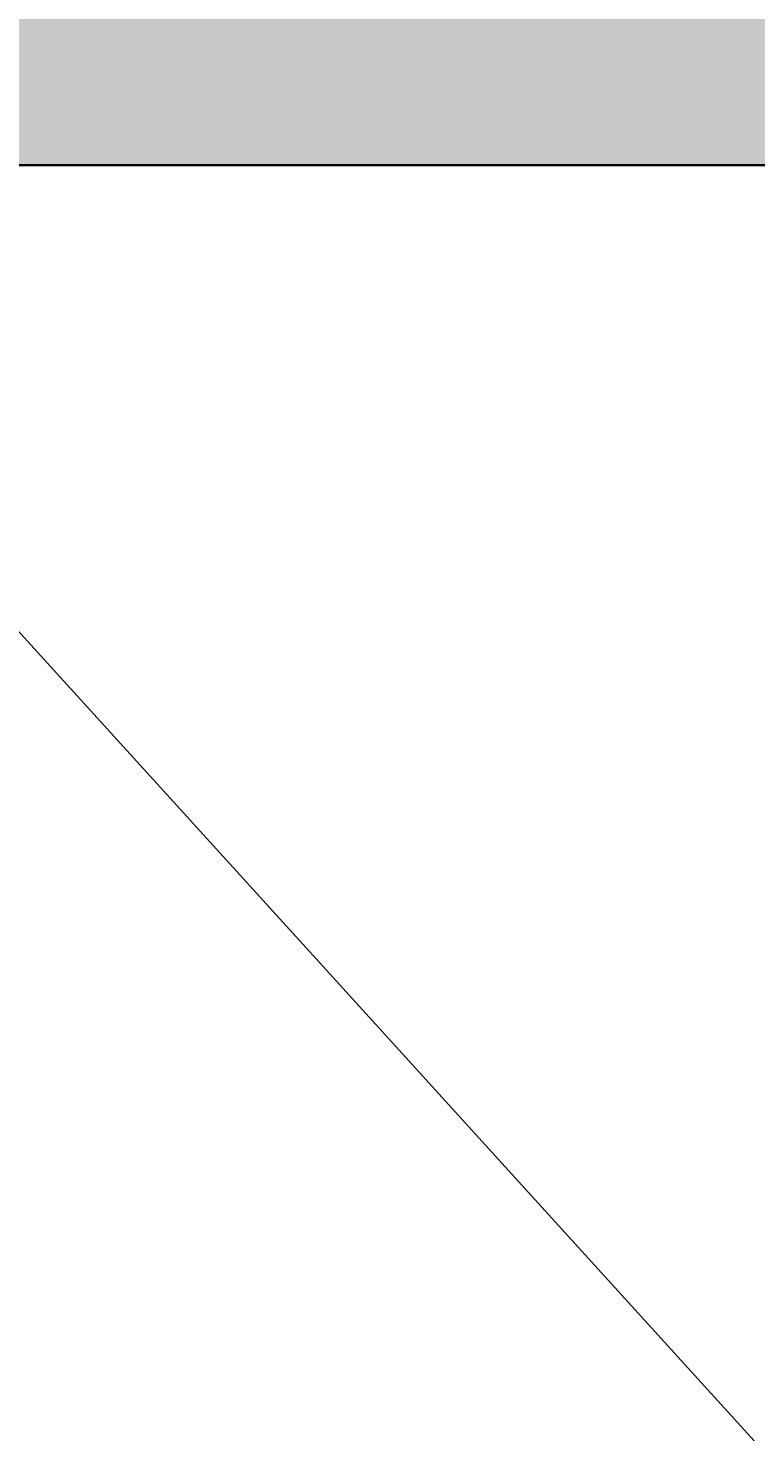
# Model space of a CAD drawing. Units: inches. Extents: x 1998 to 2588, y 1139 to 1977.
# Tile 34 of 134: x 2238 to 2257, y 1557 to 1592. Entities that reach past the tile are written whole.
import ezdxf

# ---------------------------------------------------------------- set-up
doc = ezdxf.new("R2010")
doc.units = ezdxf.units.IN
for name, color, linetype, lineweight in [('A-ANNO-DIMS', 2, 'Continuous', 18), ('A-FLOR-OPEN', 8, 'Continuous', 18), ('A-WALL-PATT', 252, 'Continuous', 13), ('WALL', 200, 'Continuous', 35)]:
    doc.layers.add(name, color=color, linetype=linetype, lineweight=lineweight)
doc.styles.get("Standard").update_dxf_attribs({"font": 'arial.ttf'})
doc.dimstyles.get("Standard").update_dxf_attribs({"dimtxt": 0.18, "dimasz": 0.18, "dimexe": 0.18, "dimexo": 0.0625, "dimgap": 0.09, "dimtad": 0, "dimtih": 1, "dimtoh": 1, "dimdec": 4, "dimzin": 0, "dimdsep": 46, "dimtxsty": 'Standard', "dimcen": 0.09, "dimadec": 0, "dimazin": 0, "dimtfac": 1, "dimtdec": 4, "dimtofl": 0, "dimtmove": 0, "dimatfit": 3, "dimfxl": 1, "dimtolj": 1, "dimtzin": 0, "dimarcsym": 0})

# ---------------------------------------------------------------- blocks, each defined once
blk = doc.blocks.new('*D34')
at = {"layer": 'A-ANNO-DIMS', "color": 0, "lineweight": -2, "transparency": 16777216}
for p, q in [((2407.91, 1594.732), (1997.843, 1594.732)), ((1998.023, 1594.552), (1998.023, 1558.913)), ((1998.023, 1522.912), (1998.023, 1558.552)), ((2407.91, 1522.732), (1997.843, 1522.732))]:
    blk.add_line(p, q, dxfattribs=at)
at = {"layer": 'A-ANNO-DIMS', "color": 0, "transparency": 16777216}
for points in [[(1997.993, 1594.552), (1998.053, 1594.552), (1998.023, 1594.732)], [(1997.993, 1522.912), (1998.053, 1522.912), (1998.023, 1522.732)]]:
    blk.add_solid(points, dxfattribs=at)
at = {"layer": 'Defpoints', "color": 0, "transparency": 16777216}
for p in [(1998.023, 1594.732), (2407.973, 1594.732), (2407.973, 1522.732)]:
    blk.add_point(p, dxfattribs=at)
at = {"layer": 'A-ANNO-DIMS', "color": 0, "transparency": 16777216, "insert": (1998.023, 1558.732), "char_height": 0.18, "attachment_point": 5}
blk.add_mtext('\\A1;72', dxfattribs=at)
blk = doc.blocks.new('*D41')
at = {"layer": 'A-ANNO-DIMS', "color": 0, "lineweight": -2, "transparency": 16777216}
for p, q in [((2227.473, 1588.67), (2227.473, 1138.602)), ((2287.473, 1588.67), (2287.473, 1138.602)), ((2227.653, 1138.782), (2257.254, 1138.782)), ((2287.293, 1138.782), (2257.692, 1138.782))]:
    blk.add_line(p, q, dxfattribs=at)
at = {"layer": 'A-ANNO-DIMS', "color": 0, "transparency": 16777216}
for points in [[(2227.653, 1138.812), (2227.653, 1138.752), (2227.473, 1138.782)], [(2287.293, 1138.812), (2287.293, 1138.752), (2287.473, 1138.782)]]:
    blk.add_solid(points, dxfattribs=at)
at = {"layer": 'Defpoints', "color": 0, "transparency": 16777216}
for p in [(2227.473, 1588.732), (2287.473, 1588.732), (2287.473, 1138.782)]:
    blk.add_point(p, dxfattribs=at)
at = {"layer": 'A-ANNO-DIMS', "color": 0, "transparency": 16777216, "insert": (2257.473, 1138.782), "char_height": 0.18, "attachment_point": 5}
blk.add_mtext('\\A1;60', dxfattribs=at)

msp = doc.modelspace()

# ---------------------------------------------------------------- hatches: boundary and pattern name
at = {"layer": 'A-WALL-PATT'}
h = msp.add_hatch(color=256, dxfattribs=at)
h.dxf.hatch_style = 1
h.paths.add_polyline_path([(2222.9729, 1888.7324), (2099.4125, 1888.7324), (2099.4125, 1879.7324), (2222.9729, 1879.7324)])
h.paths.add_polyline_path([(2096.9729, 1868.3278), (2087.9729, 1868.3278), (2087.9729, 1775.637), (2096.9729, 1775.637)])
h.paths.add_polyline_path([(2227.4729, 1868.3278), (2222.9729, 1868.3278), (2222.9729, 1774.3318), (2227.4729, 1774.3318)])
h.paths.add_polyline_path([(2188.3019, 1759.7324), (2138.6074, 1759.7324), (2099.4125, 1759.7324), (2099.4125, 1755.2324), (2176.9729, 1755.2324), (2188.3019, 1755.2324)])
h.paths.add_polyline_path([(2087.9729, 1759.7324), (2059.4729, 1759.7324), (2059.4729, 1702.7324), (2087.9729, 1702.7324), (2087.9729, 1707.2324), (2063.9729, 1707.2324), (2063.9729, 1755.2324), (2087.9729, 1755.2324)])
h.paths.add_polyline_path([(2096.9729, 1755.2324), (2087.9729, 1755.2324), (2087.9729, 1707.2324), (2096.9729, 1707.2324)])
h.paths.add_polyline_path([(2187.0461, 1707.2324), (2105.9729, 1707.2324), (2096.9729, 1707.2324), (2087.9729, 1707.2324), (2087.9729, 1702.7324), (2105.9729, 1702.7324), (2114.9729, 1702.7324), (2187.0461, 1702.7324)])
h.paths.add_polyline_path([(2181.4729, 1719.2028), (2176.9729, 1719.2028), (2176.9729, 1707.2324), (2181.4729, 1707.2324)])
h.paths.add_polyline_path([(2216.0332, 1588.7324), (2114.9729, 1588.7324), (2105.9729, 1588.7324), (2105.9729, 1584.2324), (2216.0332, 1584.2324)])
h.paths.add_polyline_path([(2077.691, 1588.7324), (2061.4729, 1588.7324), (2061.4729, 1584.2324), (2077.691, 1584.2324)])
h.paths.add_polyline_path([(2105.9729, 1588.7324), (2098.0956, 1588.7324), (2098.0956, 1584.2324), (2105.9729, 1584.2324)])
h.paths.add_polyline_path([(2114.9729, 1596.2642), (2110.1012, 1596.2642), (2105.9729, 1596.2642), (2105.9729, 1588.7324), (2114.9729, 1588.7324)])
h.paths.add_polyline_path([(2114.9729, 1584.2324), (2105.9729, 1584.2324), (2105.9729, 1580.249), (2110.1012, 1580.249), (2114.9729, 1580.249)])
h.paths.add_polyline_path([(2114.9729, 1547.7716), (2110.1012, 1547.7716, -0.0318759), (2105.9729, 1548.035), (2105.9729, 1470.2324), (2108.3775, 1470.2324), (2108.3775, 1465.7324), (2186.2943, 1465.7324), (2186.2943, 1470.2324), (2114.9729, 1470.2324)])
h.paths.add_polyline_path([(2227.4729, 1584.2324), (2222.9729, 1584.2324), (2222.9729, 1486.137), (2227.4729, 1486.137)])
h.paths.add_polyline_path([(2295.4138, 1593.2324), (2227.4729, 1593.2324), (2227.4729, 1588.7324), (2295.4138, 1588.7324), (2295.4138, 1591.8729)])
h.paths.add_polyline_path([(2345.9729, 1627.1165), (2341.4729, 1627.1165), (2341.4729, 1593.2324), (2337.2869, 1593.2324), (2337.2869, 1591.8729), (2337.2869, 1588.7324), (2345.9729, 1588.7324)])
h.paths.add_polyline_path([(2291.9729, 1588.7324), (2287.4729, 1588.7324), (2287.4729, 1522.7324), (2291.9729, 1522.7324)])
h.paths.add_polyline_path([(2291.9729, 1522.7324), (2287.4729, 1522.7324), (2227.4729, 1522.7324), (2227.4729, 1518.2324), (2291.9729, 1518.2324)])
h.paths.add_polyline_path([(2295.7347, 1519.5919), (2295.7347, 1522.7324), (2291.9729, 1522.7324), (2291.9729, 1518.2324), (2295.7347, 1518.2324)])
h.paths.add_polyline_path([(2345.9729, 1522.7324), (2337.6078, 1522.7324), (2337.6078, 1519.5919), (2337.6078, 1518.2324), (2341.4729, 1518.2324), (2341.4729, 1488.5616), (2345.9729, 1488.5616)])
h.paths.add_polyline_path([(2345.9729, 1468.1569), (2341.4729, 1468.1569), (2341.4729, 1374.2324), (2227.4729, 1374.2324), (2227.4729, 1369.7324), (2345.9729, 1369.7324)])
h.paths.add_polyline_path([(2345.9729, 1369.7324), (2341.4729, 1369.7324), (2341.4729, 1362.2324), (2345.9729, 1362.2324)])
h.paths.add_polyline_path([(2345.9729, 1317.7324), (2345.9729, 1322.2324), (2341.4729, 1322.2324), (2341.4729, 1285.137), (2345.9729, 1285.137)], flags=17)
h.paths.add_polyline_path([(2356.2096, 1322.2324), (2345.9729, 1322.2324), (2345.9729, 1317.7324), (2356.2096, 1317.7324), (2356.2096, 1319.3088)], flags=17)
h.paths.add_polyline_path([(2393.9729, 1322.2324), (2375.6999, 1322.2324), (2375.6999, 1319.3088, -0.0202458), (2375.636, 1317.7324), (2393.9729, 1317.7324)], flags=17)
h.paths.add_polyline_path([(2398.4729, 1322.2324), (2393.9729, 1322.2324), (2393.9729, 1317.7324), (2393.9729, 1237.7324), (2345.9729, 1237.7324), (2345.9729, 1264.7324), (2341.4729, 1264.7324), (2341.4729, 1228.7324), (2393.9729, 1228.7324), (2482.7412, 1228.7324), (2482.7412, 1237.7324), (2398.4729, 1237.7324), (2398.4729, 1297.1029)])
h.paths.add_polyline_path([(2398.4729, 1362.2324), (2393.9729, 1362.2324), (2393.9729, 1357.7324), (2398.4729, 1357.7324)])
h.paths.add_polyline_path([(2345.9729, 1329.7549), (2341.4729, 1329.7549), (2341.4729, 1322.2324), (2345.9729, 1322.2324)])

# ---------------------------------------------------------------- linework, layer by layer
at = {"layer": 'A-FLOR-OPEN'}
msp.add_line((2227.4729, 1588.7324), (2287.4729, 1522.7324), dxfattribs=at)
at = {"layer": 'WALL'}
msp.add_line((2295.4138, 1588.7324), (2227.4729, 1588.7324), dxfattribs=at)

# ---------------------------------------------------------------- dimensions: what is measured, and where the dimension line sits
at = {"layer": 'A-ANNO-DIMS'}
dim = msp.add_linear_dim(base=(1998.0229, 1594.7324), p1=(2407.9729, 1522.7324), p2=(2407.9729, 1594.7324), angle=90, dimstyle='Standard', override={"dimdec": 0, "dimlfac": 1, "dimrnd": 0, "dimzin": 0, "dimdsep": 46, "dimlunit": 2}, dxfattribs=at)
dim.commit()
dim.dimension.update_dxf_attribs({"geometry": '*D34', "text_midpoint": (1998.0229, 1558.7324)})
dim = msp.add_linear_dim(base=(2287.4729, 1138.7824), p1=(2227.4729, 1588.7324), p2=(2287.4729, 1588.7324), dimstyle='Standard', override={"dimdec": 0, "dimlfac": 1, "dimrnd": 0, "dimzin": 0, "dimdsep": 46, "dimlunit": 2}, dxfattribs=at)
dim.commit()
dim.dimension.update_dxf_attribs({"geometry": '*D41', "text_midpoint": (2257.4729, 1138.7824)})

doc.saveas('drawing.dxf')
